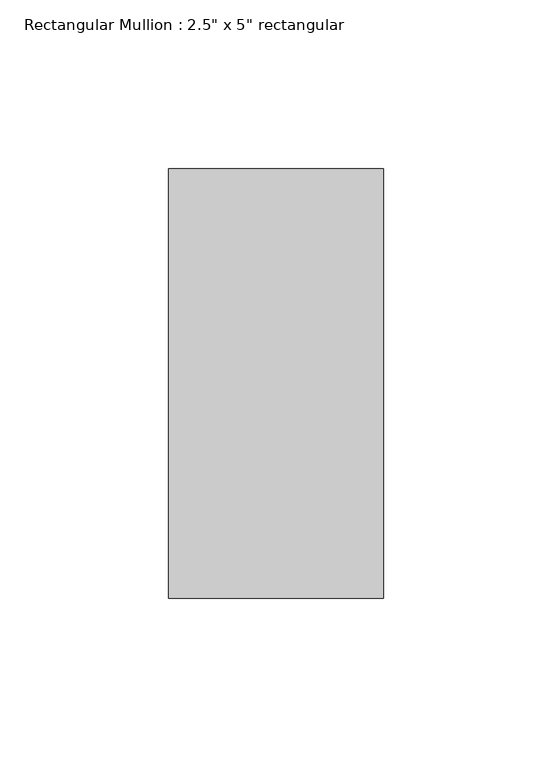
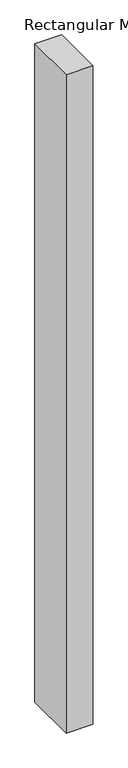
"""IFC4 building model written with IfcOpenShell, lengths in millimetres: member geometry."""

from ifc_helpers import new_model, si_unit, frame, origin, place, context, project, spatial, polyline, outline, extrude, source, transform, mapped, element, save


def member_6494088e(model_context):
    return source(origin(), model_context, "Body", "SweptSolid", [
        extrude(outline(polyline([(31.75, 63.5), (31.75, -63.5), (-31.75, -63.5), (-31.75, 63.5), (31.75, 63.5)])), frame((0.0, 0.0, -1640.1839946), z_axis=(0.0, 0.0, 1.0), x_axis=(1.0, 0.0, 0.0)), (0.0, 0.0, 1.0), 1640.1839946),
    ])


if __name__ == "__main__":
    model = new_model("IFC4")
    model_context = context("Model", 3, world=origin())
    ifc_project = project(units=[si_unit("LENGTHUNIT", "METRE", prefix="MILLI")], contexts=[model_context])
    site = spatial("IfcSite", under=ifc_project)
    building = spatial("IfcBuilding", under=site)
    placement = place(None, origin())
    member_shape = member_6494088e(model_context)
    element("IfcMember", 1, ObjectType="Rectangular Mullion : 2.5\" x 5\" rectangular", at=placement, inside=building, context=model_context, shape_type="MappedRepresentation", body=[
        mapped(member_shape, transform((0.0, 0.0, 0.0), x_axis=(1.0, 0.0, 0.0), y_axis=(0.0, 1.0, 0.0), z_axis=(0.0, 0.0, 1.0))),
    ])
    save(model, "model.ifc")

# Revit data of these elements
# Type "Rectangular Mullion : 2.5\" x 5\" rectangular"
#   built-in parameter 1007304 = 0.416667 (stored number, unit not read)
#   built-in parameter 1007301 = 0.104167 (stored number, unit not read)
#   built-in parameter 1007300 = 0.104167 (stored number, unit not read)
# Element 1 (IfcMember, "Rectangular Mullion : 2.5\" x 5\" rectangular")
#   Materials on its faces: "Aluminum"
# Materials
#   "Aluminum": class "Metal", colour RGB 247 247 247, transparency 0, Description = "Aluminum 6061", Cost = 0
